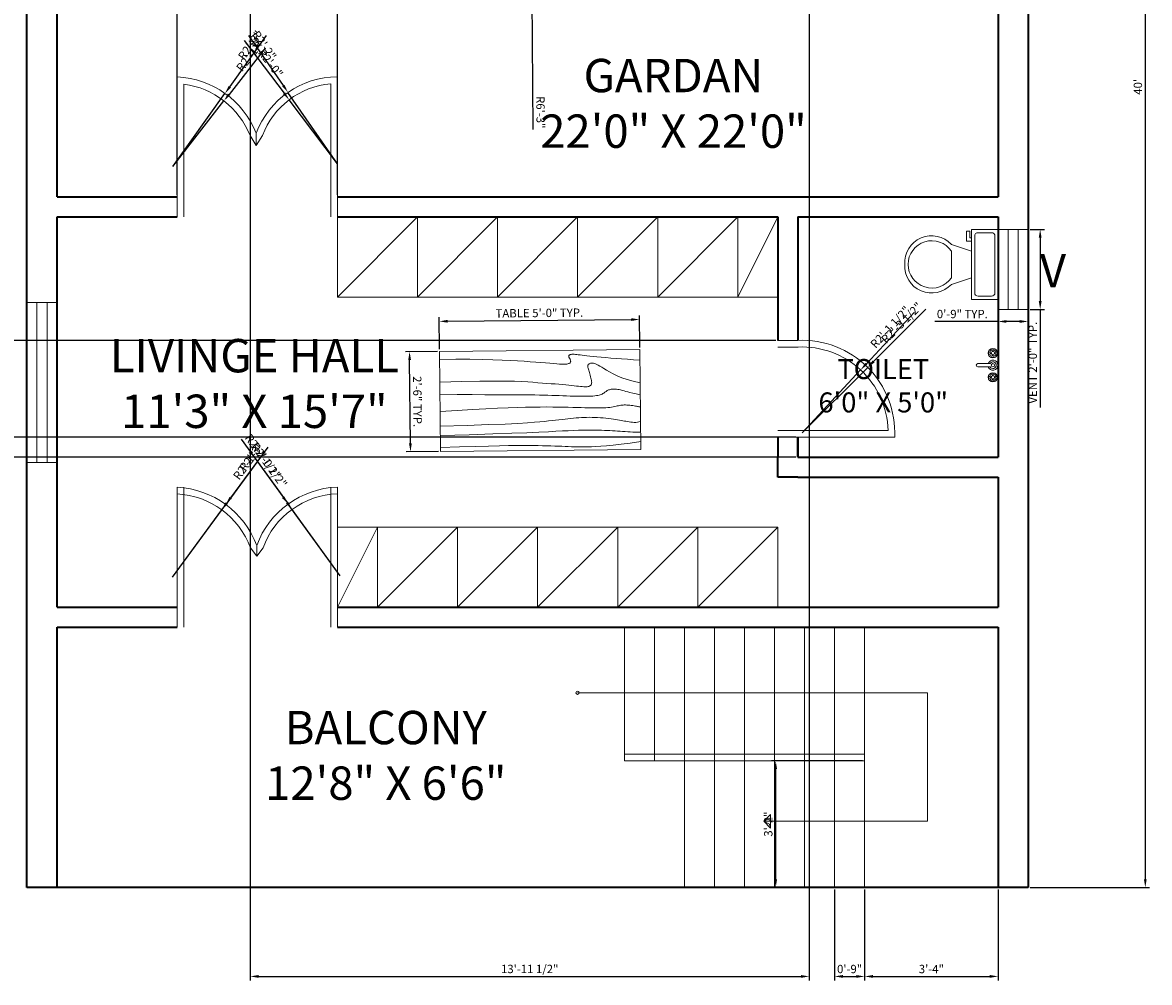
# Model space of a CAD drawing. Units: inches. Extents: x 2318 to 3542, y 1525 to 2117.
# Tile 5 of 6: x 3169 to 3507, y 1529 to 1816. Entities that reach past the tile are written whole.
import ezdxf

# ---------------------------------------------------------------- set-up
doc = ezdxf.new("R2010")
doc.units = ezdxf.units.IN
for name, color, linetype, lineweight in [('A-ANNO-DIMS', 2, 'Continuous', 18), ('A-ANNO-SYMB', 2, 'Continuous', 13), ('A-ANNO-TEXT', 7, 'Continuous', 18), ('A-AREA-IDEN', 7, 'Continuous', 25), ('A-DOOR', 4, 'Continuous', 18), ('A-FLOR-FIXT', 9, 'Continuous', 18), ('A-FLOR-STRS', 3, 'Continuous', 18), ('A-FURN', 8, 'Continuous', 18), ('A-GLAZ', 4, 'Continuous', 18), ('A-WALL', 7, 'Continuous', 35)]:
    doc.layers.add(name, color=color, linetype=linetype, lineweight=lineweight)
doc.styles.add('Annotative', font='arial.ttf')
doc.styles.get("Standard").update_dxf_attribs({"font": 'arial.ttf'})
doc.dimstyles.new('ISO-25', dxfattribs={"dimtxt": 2.5, "dimasz": 2.5, "dimexe": 1.25, "dimexo": 0.625, "dimtad": 1, "dimdec": 0, "dimlunit": 3, "dimtxsty": 'Standard', "dimcen": 2.5, "dimadec": 0, "dimazin": 0, "dimtfac": 1, "dimtdec": 0, "dimtmove": 0, "dimatfit": 3, "dimfxl": 1, "dimarcsym": 0})

# ---------------------------------------------------------------- blocks, each defined once
blk = doc.blocks.new('*D20')
at = {"layer": 'A-ANNO-DIMS', "color": 0, "lineweight": -2, "transparency": 16777216}
for p, q in [((3471.06, 2037.09), (3506.78, 2037.09)), ((3505.53, 2034.59), (3505.53, 1559.59)), ((3471.06, 1557.09), (3506.78, 1557.09))]:
    blk.add_line(p, q, dxfattribs=at)
at = {"layer": 'A-ANNO-DIMS', "color": 0, "transparency": 16777216}
for points in [[(3505.11, 2034.59), (3505.94, 2034.59), (3505.53, 2037.09)], [(3505.11, 1559.59), (3505.94, 1559.59), (3505.53, 1557.09)]]:
    blk.add_solid(points, dxfattribs=at)
at = {"layer": 'Defpoints', "color": 0, "transparency": 16777216}
for p in [(3470.43, 2037.09), (3470.43, 1557.09), (3505.53, 1557.09)]:
    blk.add_point(p, dxfattribs=at)
at = {"layer": 'A-ANNO-DIMS', "color": 0, "transparency": 16777216, "insert": (3503.63, 1797.09), "char_height": 2.5, "attachment_point": 5, "rotation": 90}
blk.add_mtext("40'", dxfattribs=at)
blk = doc.blocks.new('Table - Rectangular Woodgrain 60 x 30 in.')
for p, q in [((0, 0), (0, -30)), ((60, 0), (0, 0)), ((60, -30), (60, 0)), ((0, -30), (60, -30))]:
    blk.add_line(p, q)
for points in [[(0, -2.4), (4.8155, -2.418), (9.0302, -2.4688), (12.709, -2.5477), (15.9167, -2.65), (18.7181, -2.7711), (21.1781, -2.9063), (23.3616, -3.0508), (25.3333, -3.2), (27.1477, -3.3495), (28.8172, -3.4958), (30.3437, -3.636), (31.7291, -3.7667), (32.9756, -3.8849), (34.0849, -3.9875), (35.059, -4.0714), (35.9, -4.1334), (36.6114, -4.1711), (37.2041, -4.1854), (37.6906, -4.1779), (38.0833, -4.15), (38.3948, -4.1034), (38.6375, -4.0396), (38.8239, -3.9602), (38.9666, -3.8667), (39.0764, -3.7608), (39.1573, -3.6448), (39.2116, -3.521), (39.2416, -3.3917), (39.2498, -3.2593), (39.2385, -3.1261), (39.21, -2.9944), (39.1666, -2.8667), (39.111, -2.7447), (39.0468, -2.6281), (38.978, -2.5163), (38.9083, -2.4083), (38.8418, -2.3035), (38.7823, -2.201), (38.7337, -2.1001), (38.7, -2), (38.6844, -1.9003), (38.6875, -1.8021), (38.7094, -1.707), (38.75, -1.6167), (38.8094, -1.5326), (38.8875, -1.4563), (38.9844, -1.3893), (39.1, -1.3333), (39.2351, -1.2896), (39.3937, -1.2583), (39.5804, -1.2396), (39.8, -1.2333), (40.057, -1.2396), (40.3562, -1.2583), (40.7023, -1.2896), (41.1, -1.3333), (41.5547, -1.3895), (42.0755, -1.4573), (42.6721, -1.5361), (43.3542, -1.625), (44.1316, -1.7233), (45.014, -1.8302), (46.0114, -1.9449), (47.1333, -2.0667), (48.3862, -2.1947), (49.7625, -2.3281), (51.2513, -2.4663), (52.8416, -2.6083), (54.5226, -2.7535), (56.2833, -2.9011), (58.1127, -3.0501), (60, -3.2)], [(0, -9.2), (6.5759, -9.0858), (11.9385, -9.0365), (16.2527, -9.0418), (19.6833, -9.0917), (22.3952, -9.1759), (24.5531, -9.2844), (26.322, -9.4069), (27.8666, -9.5333), (29.3241, -9.6553), (30.7203, -9.7719), (32.0532, -9.8837), (33.3208, -9.9917), (34.5213, -10.0965), (35.6526, -10.199), (36.7128, -10.2999), (37.7, -10.4), (38.6129, -10.4996), (39.4531, -10.5969), (40.223, -10.6895), (40.925, -10.775), (41.5613, -10.8512), (42.1344, -10.9156), (42.6465, -10.966), (43.1, -11), (43.4976, -11.0158), (43.8437, -11.0136), (44.143, -10.9942), (44.4, -10.9583), (44.6195, -10.9069), (44.8062, -10.8406), (44.9648, -10.7603), (45.1, -10.6667), (45.2155, -10.5598), (45.3114, -10.4365), (45.3871, -10.2929), (45.4416, -10.125), (45.4743, -9.929), (45.4844, -9.7011), (45.4709, -9.4371), (45.4333, -9.1333), (45.3716, -8.7883), (45.2896, -8.4104), (45.1919, -8.0107), (45.0833, -7.6), (44.9685, -7.1893), (44.8521, -6.7896), (44.7388, -6.4117), (44.6333, -6.0667), (44.54, -5.7628), (44.4614, -5.4979), (44.4001, -5.2675), (44.3583, -5.0667), (44.3384, -4.8909), (44.3427, -4.7354), (44.3736, -4.5956), (44.4333, -4.4667), (44.5236, -4.3453), (44.6427, -4.2333), (44.7884, -4.1339), (44.9583, -4.05), (45.1501, -3.9849), (45.3614, -3.9417), (45.59, -3.9234), (45.8333, -3.9333), (46.0915, -3.9749), (46.3734, -4.0531), (46.6906, -4.1736), (47.0542, -4.3417), (47.4756, -4.5629), (47.9661, -4.8427), (48.5372, -5.1866), (49.2, -5.6), (49.9676, -6.0844), (50.8594, -6.625), (51.8965, -7.2031), (53.1, -7.8), (54.491, -8.3969), (56.0906, -8.975), (57.9199, -9.5156), (60, -10)], [(0, -12.8), (5.1847, -12.9322), (9.6213, -13.0323), (13.3963, -13.1059), (16.5958, -13.1583), (19.3063, -13.1952), (21.614, -13.2219), (23.6054, -13.2439), (25.3666, -13.2667), (26.9728, -13.2947), (28.4531, -13.3281), (29.8256, -13.3663), (31.1083, -13.4083), (32.3191, -13.4535), (33.476, -13.501), (34.597, -13.5501), (35.7, -13.6), (36.7984, -13.6497), (37.8875, -13.6979), (38.9578, -13.743), (40, -13.7833), (41.0047, -13.8174), (41.9625, -13.8438), (42.864, -13.8607), (43.7, -13.8667), (44.4631, -13.8604), (45.1552, -13.8417), (45.7801, -13.8104), (46.3416, -13.7667), (46.8439, -13.7104), (47.2906, -13.6417), (47.6858, -13.5604), (48.0333, -13.4667), (48.3375, -13.3608), (48.6042, -13.2448), (48.8396, -13.121), (49.05, -12.9917), (49.2417, -12.8593), (49.4208, -12.7261), (49.5937, -12.5944), (49.7667, -12.4667), (49.9452, -12.3451), (50.1323, -12.2313), (50.3303, -12.1268), (50.5416, -12.0333), (50.7686, -11.9524), (51.0135, -11.8854), (51.2788, -11.8341), (51.5666, -11.8), (51.8785, -11.7843), (52.2116, -11.7865), (52.562, -11.8059), (52.926, -11.8417), (53.2998, -11.8931), (53.6795, -11.9594), (54.0614, -12.0397), (54.4416, -12.1333), (54.8223, -12.2401), (55.2293, -12.3625), (55.6942, -12.5037), (56.2489, -12.6667), (56.9251, -12.8547), (57.7545, -13.0708), (58.7689, -13.3182), (60, -13.6)], [(0, -18), (5.124, -17.7273), (9.6609, -17.5057), (13.6705, -17.3303), (17.2125, -17.1958), (20.3467, -17.0973), (23.1328, -17.0297), (25.6307, -16.9878), (27.9, -16.9667), (29.9928, -16.9617), (31.9302, -16.9703), (33.7254, -16.9907), (35.3917, -17.0208), (36.9423, -17.0588), (38.3906, -17.1026), (39.7499, -17.1503), (41.0333, -17.2), (42.2519, -17.2496), (43.4073, -17.2969), (44.4986, -17.3395), (45.525, -17.375), (46.4858, -17.4012), (47.3802, -17.4156), (48.2074, -17.416), (48.9667, -17.4), (49.6583, -17.3662), (50.2872, -17.3167), (50.8595, -17.2547), (51.3812, -17.1833), (51.8584, -17.1057), (52.2971, -17.025), (52.7034, -16.9443), (53.0833, -16.8667), (53.443, -16.7951), (53.789, -16.7313), (54.128, -16.6768), (54.4666, -16.6334), (54.8115, -16.6024), (55.1693, -16.5854), (55.5465, -16.5841), (55.95, -16.6), (56.3828, -16.6337), (56.8346, -16.6823), (57.2915, -16.7418), (57.7396, -16.8084), (58.165, -16.878), (58.5539, -16.9469), (58.8924, -17.0111), (59.1666, -17.0667), (59.3679, -17.1107), (59.5078, -17.1438), (59.6032, -17.1675), (59.6708, -17.1833), (59.7275, -17.193), (59.7901, -17.1979), (59.8753, -17.1998), (60, -17.2)], [(0, -22.4), (8.0098, -22.2501), (14.4094, -22.1011), (19.4168, -21.9535), (23.25, -21.8083), (26.1269, -21.6663), (28.2656, -21.5281), (29.884, -21.3947), (31.2, -21.2667), (32.3967, -21.1448), (33.5172, -21.0292), (34.5697, -20.9198), (35.5625, -20.8167), (36.5037, -20.7198), (37.4015, -20.6292), (38.2642, -20.5448), (39.1, -20.4667), (39.9164, -20.3951), (40.7187, -20.3313), (41.5117, -20.2768), (42.3, -20.2333), (43.0883, -20.2024), (43.8812, -20.1854), (44.6836, -20.1841), (45.5, -20.2), (46.3328, -20.234), (47.1747, -20.2844), (48.0163, -20.3488), (48.8479, -20.425), (49.66, -20.5106), (50.4429, -20.6031), (51.1872, -20.7004), (51.8833, -20.8), (52.5246, -20.8999), (53.1166, -20.9995), (53.6681, -21.0983), (54.1875, -21.1958), (54.6834, -21.2919), (55.1646, -21.3859), (55.6394, -21.4777), (56.1167, -21.5667), (56.6028, -21.6515), (57.0961, -21.7266), (57.5929, -21.7852), (58.0896, -21.8208), (58.5823, -21.8268), (59.0674, -21.7964), (59.5412, -21.723), (60, -21.6)], [(0, -25.2), (8.6355, -25.0504), (15.7026, -24.9031), (21.4049, -24.7606), (25.9458, -24.625), (29.529, -24.4988), (32.3578, -24.3844), (34.6359, -24.284), (36.5667, -24.2), (38.3213, -24.1341), (39.9417, -24.0854), (41.437, -24.0523), (42.8167, -24.0333), (44.0901, -24.0268), (45.2667, -24.0313), (46.3557, -24.0451), (47.3667, -24.0667), (48.309, -24.0947), (49.1928, -24.1287), (50.0284, -24.168), (50.826, -24.2125), (51.5959, -24.2617), (52.3483, -24.3151), (53.0935, -24.3725), (53.8417, -24.4334), (54.6009, -24.497), (55.3699, -24.561), (56.1454, -24.6226), (56.9239, -24.6792), (57.7021, -24.7279), (58.4764, -24.7662), (59.2435, -24.7911), (60, -24.8)], [(0, -28.8), (5.6867, -28.6681), (10.45, -28.5698), (14.407, -28.5012), (17.675, -28.4584), (20.3711, -28.4374), (22.6125, -28.4344), (24.5164, -28.4455), (26.2, -28.4667), (27.762, -28.4947), (29.2276, -28.5281), (30.6033, -28.5663), (31.8958, -28.6084), (33.1118, -28.6535), (34.2578, -28.7011), (35.3405, -28.7501), (36.3666, -28.8), (37.3443, -28.8497), (38.288, -28.8974), (39.2137, -28.9412), (40.1375, -28.9792), (41.0753, -29.0093), (42.0432, -29.0297), (43.0572, -29.0384), (44.1333, -29.0333), (45.2936, -29.0114), (46.5843, -28.9641), (48.0579, -28.8816), (49.7666, -28.7542), (51.7629, -28.5721), (54.0989, -28.3255), (56.8272, -28.0048), (60, -27.6)]]:
    blk.add_lwpolyline(points)
blk = doc.blocks.new('*U14')
for p, q in [((241.3, -152.4), (241.3, -50.8)), ((-254, -215.9), (-203.2, -215.9)), ((-254, -241.3), (-254, -215.9)), ((-177.8, -241.3), (-254, -241.3)), ((-203.2, -215.9), (-203.2, -203.2)), ((-177.8, -203.2), (-177.8, -241.3)), ((-101.6, -203.2), (-152.4, -355.6)), ((101.6, -203.2), (152.4, -355.6)), ((101.6, -355.6), (-101.6, -355.6))]:
    blk.add_line(p, q)
blk.add_lwpolyline([(266.7, -203.2), (266.7, 0), (-266.7, 0), (-266.7, -203.2)], close=True)
for points in [[(-241.3, -50.8), (-241.3, -152.4)], [(215.9, -25.4), (-215.9, -25.4)], [(-215.9, -177.8), (215.9, -177.8)]]:
    blk.add_lwpolyline(points)
for centre, radius, start, end in [((-219.075, -47.625), 22.45064, 81.8699, 188.1301), ((219.075, -47.625), 22.45064, 351.8699, 98.1301), ((-219.075, -155.575), 22.45064, 171.869898, 278.1301), ((219.075, -155.575), 22.45064, 261.8699, 8.1301), ((-12.12088, -505.93752), 205.61935, 133.01722, 273.38), ((0.94996, -504.77674), 181.02486, 124.50543, 269.7), ((-0.94742, -504.77674), 181.02486, 270.3, 55.4946), ((12.12342, -505.93752), 205.61935, 266.62, 46.9828)]:
    blk.add_arc(centre, radius, start, end)
blk = doc.blocks.new('Faucet - Bathroom top')
for p, q in [((-4.107, 0.125), (-4.375, 0.125)), ((-3.75, 0.4788), (-3.75, 0.75)), ((-3.5, 0.482), (-3.5, 0.75)), ((-3.1461, 0.125), (-2.875, 0.125)), ((3.143, 0.125), (2.875, 0.125)), ((3.5, 0.4788), (3.5, 0.75)), ((3.75, 0.482), (3.75, 0.75)), ((4.1039, 0.125), (4.375, 0.125)), ((-4.1039, -0.125), (-4.375, -0.125)), ((-3.75, -0.4821), (-3.75, -0.75)), ((-3.5, -0.4789), (-3.5, -0.75)), ((-3.143, -0.125), (-2.875, -0.125)), ((-0.5, -0.8639), (-0.5, -4.5)), ((0.5, -4.5), (0.5, -0.8631)), ((3.1461, -0.125), (2.875, -0.125)), ((3.5, -0.4821), (3.5, -0.75)), ((3.75, -0.4789), (3.75, -0.75)), ((4.107, -0.125), (4.375, -0.125))]:
    blk.add_line(p, q)
for centre, radius in [((-3.625, 0), 1.375), ((-4.625, 0), 0.2795), ((-3.625, 0), 0.5), ((-3.625, 1), 0.2795), ((-2.625, 0), 0.2795), ((0, 0), 0.5), ((3.625, 0), 1.375), ((2.625, 0), 0.2795), ((3.625, 0), 0.5), ((3.625, 1), 0.2795), ((4.625, 0), 0.2795), ((-3.625, -1), 0.2795), ((3.625, -1), 0.2795)]:
    blk.add_circle(centre, radius)
for centre, radius, start, end in [((-3.625, 0), 1, 105.2407, 164.2093), ((-3.625, 0), 1, 16.44125, 74.07887), ((0, 0), 1.5, 289.6514, 250.3603), ((0, 0), 1, 300.3431, 239.7554), ((3.625, 0), 1, 106.12, 164.0884), ((3.625, 0), 1, 16.23422, 73.90469), ((-3.625, 0), 1, 196.2342, 253.9047), ((-3.625, 0), 1, 286.12, 344.0884), ((3.625, 0), 1, 196.4413, 254.0789), ((3.625, 0), 1, 285.2407, 344.2093), ((0, -4.5), 0.5, 180, 0)]:
    blk.add_arc(centre, radius, start, end)
blk = doc.blocks.new('WIN-48x9')
for p, q in [((48, 9), (0, 9)), ((0, 9), (0, 0)), ((48, 0), (48, 9)), ((48, 6), (0, 6)), ((0, 3), (48, 3)), ((0, 0), (48, 0))]:
    blk.add_line(p, q)
blk = doc.blocks.new('VENT-24x9')
for p, q in [((0, 24), (0, 0)), ((9, 24), (0, 24)), ((3, 24), (3, 0)), ((6, 0), (6, 24)), ((9, 0), (9, 24)), ((0, 0), (9, 0))]:
    blk.add_line(p, q)
blk = doc.blocks.new('STAIR-ARROWHEAD')
for p, q in [((0, 2), (2, 4)), ((2, 2), (2, 4)), ((2, 4), (2, 2)), ((2, 4), (2, 0)), ((0, 2), (2, 3)), ((2, 2), (0, 2)), ((2, 0), (0, 2)), ((2, 1), (0, 2)), ((2, 3), (2, 1)), ((2, 2), (2, 0)), ((2, 0), (2, 2))]:
    blk.add_line(p, q)
blk = doc.blocks.new('*D34')
at = {"layer": 'A-ANNO-DIMS', "color": 0, "lineweight": -2, "transparency": 16777216}
for p, q in [((3471.06, 1754.36), (3475.28, 1754.36)), ((3474.03, 1751.86), (3474.03, 1732.86)), ((3471.06, 1730.36), (3475.28, 1730.36)), ((3474.03, 1730.36), (3474.03, 1700.96))]:
    blk.add_line(p, q, dxfattribs=at)
at = {"layer": 'A-ANNO-DIMS', "color": 0, "transparency": 16777216}
for points in [[(3473.61, 1751.86), (3474.45, 1751.86), (3474.03, 1754.36)], [(3473.61, 1732.86), (3474.45, 1732.86), (3474.03, 1730.36)]]:
    blk.add_solid(points, dxfattribs=at)
at = {"layer": 'Defpoints', "color": 0, "transparency": 16777216}
for p in [(3470.43, 1754.36), (3470.43, 1730.36), (3474.03, 1730.36)]:
    blk.add_point(p, dxfattribs=at)
at = {"layer": 'A-ANNO-DIMS', "color": 0, "transparency": 16777216, "insert": (3472.13, 1714.41), "char_height": 2.5, "attachment_point": 5, "rotation": 90}
blk.add_mtext('VENT 2\'-0" TYP.', dxfattribs=at)
blk = doc.blocks.new('*D35')
at = {"layer": 'A-ANNO-DIMS', "color": 0, "lineweight": -2, "transparency": 16777216}
for p, q in [((3461.43, 1729.74), (3461.43, 1725.51)), ((3470.43, 1729.74), (3470.43, 1725.51)), ((3461.43, 1726.76), (3442.44, 1726.76)), ((3467.93, 1726.76), (3463.93, 1726.76))]:
    blk.add_line(p, q, dxfattribs=at)
at = {"layer": 'A-ANNO-DIMS', "color": 0, "transparency": 16777216}
for points in [[(3463.93, 1727.18), (3463.93, 1726.35), (3461.43, 1726.76)], [(3467.93, 1727.18), (3467.93, 1726.35), (3470.43, 1726.76)]]:
    blk.add_solid(points, dxfattribs=at)
at = {"layer": 'Defpoints', "color": 0, "transparency": 16777216}
for p in [(3461.43, 1730.36), (3470.43, 1730.36), (3461.43, 1726.76)]:
    blk.add_point(p, dxfattribs=at)
at = {"layer": 'A-ANNO-DIMS', "color": 0, "transparency": 16777216, "insert": (3450.69, 1728.67), "char_height": 2.5, "attachment_point": 5}
blk.add_mtext('0\'-9" TYP.', dxfattribs=at)
blk = doc.blocks.new('*D44')
at = {"layer": 'A-ANNO-DIMS', "color": 0, "lineweight": -2, "transparency": 16777216}
for p, q in [((3294.06, 1718.42), (3293.97, 1728.05)), ((3296.48, 1726.82), (3351.48, 1727.33)), ((3354.06, 1718.98), (3353.97, 1728.6))]:
    blk.add_line(p, q, dxfattribs=at)
at = {"layer": 'A-ANNO-DIMS', "color": 0, "transparency": 16777216}
for points in [[(3296.48, 1727.24), (3296.49, 1726.4), (3293.98, 1726.8)], [(3351.48, 1727.75), (3351.48, 1726.91), (3353.98, 1727.35)]]:
    blk.add_solid(points, dxfattribs=at)
at = {"layer": 'Defpoints', "color": 0, "transparency": 16777216}
for p in [(3353.98, 1727.35), (3294.07, 1717.8), (3354.06, 1718.35)]:
    blk.add_point(p, dxfattribs=at)
at = {"layer": 'A-ANNO-DIMS', "color": 0, "transparency": 16777216, "insert": (3323.96, 1728.98), "char_height": 2.5, "attachment_point": 5, "rotation": 0.5327}
blk.add_mtext('TABLE 5\'-0" TYP.', dxfattribs=at)
blk = doc.blocks.new('*D45')
at = {"layer": 'A-ANNO-DIMS', "color": 0, "lineweight": -2, "transparency": 16777216}
for p, q in [((3293.44, 1717.79), (3283.82, 1717.7)), ((3285.32, 1690.21), (3285.09, 1715.21)), ((3293.72, 1687.79), (3284.1, 1687.7))]:
    blk.add_line(p, q, dxfattribs=at)
at = {"layer": 'A-ANNO-DIMS', "color": 0, "transparency": 16777216}
for points in [[(3285.51, 1715.22), (3284.67, 1715.21), (3285.07, 1717.71)], [(3285.74, 1690.22), (3284.91, 1690.21), (3285.35, 1687.71)]]:
    blk.add_solid(points, dxfattribs=at)
at = {"layer": 'Defpoints', "color": 0, "transparency": 16777216}
for p in [(3285.07, 1717.71), (3294.07, 1717.8), (3294.35, 1687.8)]:
    blk.add_point(p, dxfattribs=at)
at = {"layer": 'A-ANNO-DIMS', "color": 0, "transparency": 16777216, "insert": (3287.11, 1702.73), "char_height": 2.5, "attachment_point": 5, "rotation": 270.5327}
blk.add_mtext('2\'-6" TYP.', dxfattribs=at)
blk = doc.blocks.new('*D53')
at = {"layer": 'A-ANNO-DIMS', "color": 0, "lineweight": -2, "transparency": 16777216}
for p, q in [((3237.33, 1838.64), (3237.33, 1529.19)), ((3404.83, 1824.73), (3404.83, 1529.19)), ((3239.83, 1530.44), (3402.33, 1530.44))]:
    blk.add_line(p, q, dxfattribs=at)
at = {"layer": 'A-ANNO-DIMS', "color": 0, "transparency": 16777216}
for points in [[(3239.83, 1530.86), (3239.83, 1530.02), (3237.33, 1530.44)], [(3402.33, 1530.86), (3402.33, 1530.02), (3404.83, 1530.44)]]:
    blk.add_solid(points, dxfattribs=at)
at = {"layer": 'Defpoints', "color": 0, "transparency": 16777216}
for p in [(3237.33, 1839.27), (3404.83, 1825.36), (3404.83, 1530.44)]:
    blk.add_point(p, dxfattribs=at)
at = {"layer": 'A-ANNO-DIMS', "color": 0, "transparency": 16777216, "insert": (3321.08, 1532.36), "char_height": 2.5, "attachment_point": 5}
blk.add_mtext('13\'-11 1/2"', dxfattribs=at)
blk = doc.blocks.new('*D61')
at = {"layer": 'A-ANNO-DIMS', "color": 0, "lineweight": -2, "transparency": 16777216}
for p, q in [((3215.43, 1764.71), (3215.43, 2114.76)), ((3263.43, 1764.71), (3263.43, 2114.76)), ((3217.93, 2113.51), (3260.93, 2113.51))]:
    blk.add_line(p, q, dxfattribs=at)
at = {"layer": 'A-ANNO-DIMS', "color": 0, "transparency": 16777216}
for points in [[(3217.93, 2113.93), (3217.93, 2113.1), (3215.43, 2113.51)], [(3260.93, 2113.93), (3260.93, 2113.1), (3263.43, 2113.51)]]:
    blk.add_solid(points, dxfattribs=at)
at = {"layer": 'Defpoints', "color": 0, "transparency": 16777216}
for p in [(3263.43, 2113.51), (3215.43, 1764.09), (3263.43, 1764.09)]:
    blk.add_point(p, dxfattribs=at)
at = {"layer": 'A-ANNO-DIMS', "color": 0, "transparency": 16777216, "insert": (3239.43, 2115.41), "char_height": 2.5, "attachment_point": 5}
blk.add_mtext('4\'-0"', dxfattribs=at)
blk = doc.blocks.new('*D64')
at = {"layer": 'A-ANNO-DIMS', "color": 0, "lineweight": -2, "transparency": 16777216}
for p, q in [((3394.81, 1721.09), (3104.01, 1721.09)), ((3105.26, 1694.59), (3105.26, 1718.59)), ((3394.81, 1692.09), (3104.01, 1692.09))]:
    blk.add_line(p, q, dxfattribs=at)
at = {"layer": 'A-ANNO-DIMS', "color": 0, "transparency": 16777216}
for points in [[(3104.85, 1718.59), (3105.68, 1718.59), (3105.26, 1721.09)], [(3104.85, 1694.59), (3105.68, 1694.59), (3105.26, 1692.09)]]:
    blk.add_solid(points, dxfattribs=at)
at = {"layer": 'Defpoints', "color": 0, "transparency": 16777216}
for p in [(3105.26, 1721.09), (3395.43, 1721.09), (3395.43, 1692.09)]:
    blk.add_point(p, dxfattribs=at)
at = {"layer": 'A-ANNO-DIMS', "color": 0, "transparency": 16777216, "insert": (3103.36, 1706.59), "char_height": 2.5, "attachment_point": 5, "rotation": 90}
blk.add_mtext('2\'-5"', dxfattribs=at)
blk = doc.blocks.new('*D65')
at = {"layer": 'A-ANNO-DIMS', "color": 0, "lineweight": -2, "transparency": 16777216}
for p, q in [((3105.26, 1694.59), (3105.26, 1704.98)), ((3400.81, 1692.09), (3104.01, 1692.09)), ((3105.26, 1686.09), (3105.26, 1692.09)), ((3400.81, 1686.09), (3104.01, 1686.09)), ((3105.26, 1683.59), (3105.26, 1681.09))]:
    blk.add_line(p, q, dxfattribs=at)
at = {"layer": 'A-ANNO-DIMS', "color": 0, "transparency": 16777216}
for points in [[(3104.85, 1694.59), (3105.68, 1694.59), (3105.26, 1692.09)], [(3104.85, 1683.59), (3105.68, 1683.59), (3105.26, 1686.09)]]:
    blk.add_solid(points, dxfattribs=at)
at = {"layer": 'Defpoints', "color": 0, "transparency": 16777216}
for p in [(3105.26, 1692.09), (3401.43, 1692.09), (3401.43, 1686.09)]:
    blk.add_point(p, dxfattribs=at)
at = {"layer": 'A-ANNO-DIMS', "color": 0, "transparency": 16777216, "insert": (3103.36, 1701.04), "char_height": 2.5, "attachment_point": 5, "rotation": 90}
blk.add_mtext('0\'-6"', dxfattribs=at)
blk = doc.blocks.new('*D68')
at = {"layer": 'A-ANNO-DIMS', "color": 0, "lineweight": -2, "transparency": 16777216}
for p, q in [((3420.81, 1595.09), (3393.53, 1595.09)), ((3394.78, 1559.59), (3394.78, 1592.59)), ((3420.81, 1557.09), (3393.53, 1557.09))]:
    blk.add_line(p, q, dxfattribs=at)
at = {"layer": 'A-ANNO-DIMS', "color": 0, "transparency": 16777216}
for points in [[(3394.36, 1592.59), (3395.2, 1592.59), (3394.78, 1595.09)], [(3394.36, 1559.59), (3395.2, 1559.59), (3394.78, 1557.09)]]:
    blk.add_solid(points, dxfattribs=at)
at = {"layer": 'Defpoints', "color": 0, "transparency": 16777216}
for p in [(3394.78, 1595.09), (3421.43, 1595.09), (3421.43, 1557.09)]:
    blk.add_point(p, dxfattribs=at)
at = {"layer": 'A-ANNO-DIMS', "color": 0, "transparency": 16777216, "insert": (3392.88, 1576.09), "char_height": 2.5, "attachment_point": 5, "rotation": 90}
blk.add_mtext('3\'-2"', dxfattribs=at)
blk = doc.blocks.new('*D69')
at = {"layer": 'A-ANNO-DIMS', "color": 0, "lineweight": -2, "transparency": 16777216}
for p, q in [((3412.43, 1556.46), (3412.43, 1529.19)), ((3421.43, 1556.46), (3421.43, 1529.19)), ((3414.93, 1530.44), (3418.93, 1530.44))]:
    blk.add_line(p, q, dxfattribs=at)
at = {"layer": 'A-ANNO-DIMS', "color": 0, "transparency": 16777216}
for points in [[(3414.93, 1530.86), (3414.93, 1530.02), (3412.43, 1530.44)], [(3418.93, 1530.86), (3418.93, 1530.02), (3421.43, 1530.44)]]:
    blk.add_solid(points, dxfattribs=at)
at = {"layer": 'Defpoints', "color": 0, "transparency": 16777216}
for p in [(3412.43, 1557.09), (3421.43, 1557.09), (3421.43, 1530.44)]:
    blk.add_point(p, dxfattribs=at)
at = {"layer": 'A-ANNO-DIMS', "color": 0, "transparency": 16777216, "insert": (3416.93, 1532.34), "char_height": 2.5, "attachment_point": 5}
blk.add_mtext('0\'-9"', dxfattribs=at)
blk = doc.blocks.new('*D70')
at = {"layer": 'A-ANNO-DIMS', "color": 0, "lineweight": -2, "transparency": 16777216}
for p, q in [((3421.43, 1556.46), (3421.43, 1529.19)), ((3461.43, 1556.46), (3461.43, 1529.19)), ((3423.93, 1530.44), (3458.93, 1530.44))]:
    blk.add_line(p, q, dxfattribs=at)
at = {"layer": 'A-ANNO-DIMS', "color": 0, "transparency": 16777216}
for points in [[(3423.93, 1530.86), (3423.93, 1530.02), (3421.43, 1530.44)], [(3458.93, 1530.86), (3458.93, 1530.02), (3461.43, 1530.44)]]:
    blk.add_solid(points, dxfattribs=at)
at = {"layer": 'Defpoints', "color": 0, "transparency": 16777216}
for p in [(3421.43, 1557.09), (3461.43, 1557.09), (3461.43, 1530.44)]:
    blk.add_point(p, dxfattribs=at)
at = {"layer": 'A-ANNO-DIMS', "color": 0, "transparency": 16777216, "insert": (3441.43, 1532.34), "char_height": 2.5, "attachment_point": 5}
blk.add_mtext('3\'-4"', dxfattribs=at)
blk = doc.blocks.new('*D86')
at = {"layer": 'A-ANNO-DIMS', "color": 0, "lineweight": -2, "transparency": 16777216}
for p, q in [((3439.8, 1730.46), (3424.11, 1714.77)), ((3402.73, 1693.39), (3422.34, 1713))]:
    blk.add_line(p, q, dxfattribs=at)
at = {"layer": 'A-ANNO-DIMS', "color": 0, "transparency": 16777216}
blk.add_solid([(3423.81, 1715.06), (3424.4, 1714.47), (3422.34, 1713)], dxfattribs=at)
at = {"layer": 'Defpoints', "color": 0, "transparency": 16777216}
for p in [(3422.34, 1713), (3402.73, 1693.39)]:
    blk.add_point(p, dxfattribs=at)
at = {"layer": 'A-ANNO-DIMS', "color": 0, "transparency": 16777216, "insert": (3432.75, 1726.12), "char_height": 2.5, "attachment_point": 5, "rotation": 45.0003}
blk.add_mtext('R2\'-3 1/2"', dxfattribs=at)
blk = doc.blocks.new('*D92')
at = {"layer": 'A-ANNO-DIMS', "color": 0, "lineweight": -2, "transparency": 16777216}
for p, q in [((3242.11, 1812.45), (3231.21, 1797.16)), ((3214.15, 1773.23), (3229.75, 1795.13))]:
    blk.add_line(p, q, dxfattribs=at)
at = {"layer": 'A-ANNO-DIMS', "color": 0, "transparency": 16777216}
blk.add_solid([(3230.87, 1797.4), (3231.55, 1796.92), (3229.75, 1795.13)], dxfattribs=at)
at = {"layer": 'Defpoints', "color": 0, "transparency": 16777216}
for p in [(3229.75, 1795.13), (3214.15, 1773.23)]:
    blk.add_point(p, dxfattribs=at)
at = {"layer": 'A-ANNO-DIMS', "color": 0, "transparency": 16777216, "insert": (3237.57, 1809.37), "char_height": 2.5, "attachment_point": 5, "rotation": 54.5145}
blk.add_mtext('R2\'-3"', dxfattribs=at)
blk = doc.blocks.new('*D93')
at = {"layer": 'A-ANNO-DIMS', "color": 0, "lineweight": -2, "transparency": 16777216}
for p, q in [((3236.79, 1812.5), (3247.22, 1797.49)), ((3263.5, 1774.04), (3248.64, 1795.44))]:
    blk.add_line(p, q, dxfattribs=at)
at = {"layer": 'A-ANNO-DIMS', "color": 0, "transparency": 16777216}
blk.add_solid([(3247.56, 1797.73), (3246.87, 1797.25), (3248.64, 1795.44)], dxfattribs=at)
at = {"layer": 'Defpoints', "color": 0, "transparency": 16777216}
for p in [(3248.64, 1795.44), (3263.5, 1774.04)]:
    blk.add_point(p, dxfattribs=at)
at = {"layer": 'A-ANNO-DIMS', "color": 0, "transparency": 16777216, "insert": (3241.27, 1809.34), "char_height": 2.5, "attachment_point": 5, "rotation": 304.7777}
blk.add_mtext('R2\'-2"', dxfattribs=at)
blk = doc.blocks.new('*D94')
at = {"layer": 'A-ANNO-DIMS', "color": 0, "lineweight": -2, "transparency": 16777216}
for p, q in [((3242.59, 1689.1), (3231.45, 1673.92)), ((3214.02, 1650.15), (3229.97, 1671.9))]:
    blk.add_line(p, q, dxfattribs=at)
at = {"layer": 'A-ANNO-DIMS', "color": 0, "transparency": 16777216}
blk.add_solid([(3231.12, 1674.17), (3231.79, 1673.67), (3229.97, 1671.9)], dxfattribs=at)
at = {"layer": 'Defpoints', "color": 0, "transparency": 16777216}
for p in [(3229.97, 1671.9), (3214.02, 1650.15)]:
    blk.add_point(p, dxfattribs=at)
at = {"layer": 'A-ANNO-DIMS', "color": 0, "transparency": 16777216, "insert": (3238.01, 1686.08), "char_height": 2.5, "attachment_point": 5, "rotation": 53.7455}
blk.add_mtext('R2\'-3"', dxfattribs=at)
blk = doc.blocks.new('*D95')
at = {"layer": 'A-ANNO-DIMS', "color": 0, "lineweight": -2, "transparency": 16777216}
for p, q in [((3234.59, 1691.48), (3247.21, 1674.07)), ((3264.27, 1650.53), (3248.68, 1672.04))]:
    blk.add_line(p, q, dxfattribs=at)
at = {"layer": 'A-ANNO-DIMS', "color": 0, "transparency": 16777216}
blk.add_solid([(3247.55, 1674.31), (3246.87, 1673.82), (3248.68, 1672.04)], dxfattribs=at)
at = {"layer": 'Defpoints', "color": 0, "transparency": 16777216}
for p in [(3248.68, 1672.04), (3264.27, 1650.53)]:
    blk.add_point(p, dxfattribs=at)
at = {"layer": 'A-ANNO-DIMS', "color": 0, "transparency": 16777216, "insert": (3240.87, 1686.08), "char_height": 2.5, "attachment_point": 5, "rotation": 305.9363}
blk.add_mtext('R2\'-2 1/2"', dxfattribs=at)
blk = doc.blocks.new('*D102')
at = {"layer": 'A-ANNO-DIMS', "color": 0, "lineweight": -2, "transparency": 16777216}
for p, q in [((3436.23, 1729.46), (3421.94, 1714.08)), ((3402.73, 1693.39), (3420.24, 1712.24))]:
    blk.add_line(p, q, dxfattribs=at)
at = {"layer": 'A-ANNO-DIMS', "color": 0, "transparency": 16777216}
blk.add_solid([(3421.63, 1714.36), (3422.25, 1713.79), (3420.24, 1712.24)], dxfattribs=at)
at = {"layer": 'Defpoints', "color": 0, "transparency": 16777216}
for p in [(3420.24, 1712.24), (3402.73, 1693.39)]:
    blk.add_point(p, dxfattribs=at)
at = {"layer": 'A-ANNO-DIMS', "color": 0, "transparency": 16777216, "insert": (3429.34, 1724.86), "char_height": 2.5, "attachment_point": 5, "rotation": 47.1232}
blk.add_mtext('R2\'-1 1/2"', dxfattribs=at)
blk = doc.blocks.new('*D103')
at = {"layer": 'A-ANNO-DIMS', "color": 0, "lineweight": -2, "transparency": 16777216}
for p, q in [((3240.7, 1686.52), (3230.27, 1672.31)), ((3214.02, 1650.15), (3228.79, 1670.29))]:
    blk.add_line(p, q, dxfattribs=at)
at = {"layer": 'A-ANNO-DIMS', "color": 0, "transparency": 16777216}
blk.add_solid([(3229.93, 1672.55), (3230.61, 1672.06), (3228.79, 1670.29)], dxfattribs=at)
at = {"layer": 'Defpoints', "color": 0, "transparency": 16777216}
for p in [(3228.79, 1670.29), (3214.02, 1650.15)]:
    blk.add_point(p, dxfattribs=at)
at = {"layer": 'A-ANNO-DIMS', "color": 0, "transparency": 16777216, "insert": (3236.14, 1683.49), "char_height": 2.5, "attachment_point": 5, "rotation": 53.7439}
blk.add_mtext('R2\'-1"', dxfattribs=at)
blk = doc.blocks.new('*D105')
at = {"layer": 'A-ANNO-DIMS', "color": 0, "lineweight": -2, "transparency": 16777216}
for p, q in [((3235.51, 1810.96), (3247.46, 1795.2)), ((3263.5, 1774.04), (3248.97, 1793.2))]:
    blk.add_line(p, q, dxfattribs=at)
at = {"layer": 'A-ANNO-DIMS', "color": 0, "transparency": 16777216}
blk.add_solid([(3247.79, 1795.45), (3247.13, 1794.94), (3248.97, 1793.2)], dxfattribs=at)
at = {"layer": 'Defpoints', "color": 0, "transparency": 16777216}
for p in [(3248.97, 1793.2), (3263.5, 1774.04)]:
    blk.add_point(p, dxfattribs=at)
at = {"layer": 'A-ANNO-DIMS', "color": 0, "transparency": 16777216, "insert": (3241.77, 1805.85), "char_height": 2.5, "attachment_point": 5, "rotation": 307.1715}
blk.add_mtext('2X R2\'-0"', dxfattribs=at)
blk = doc.blocks.new('*D112')
at = {"layer": 'A-ANNO-DIMS', "color": 0, "lineweight": -2, "transparency": 16777216}
for p, q in [((3241.77, 1808.71), (3230.97, 1794.84)), ((3214.15, 1773.23), (3229.44, 1792.87))]:
    blk.add_line(p, q, dxfattribs=at)
at = {"layer": 'A-ANNO-DIMS', "color": 0, "transparency": 16777216}
blk.add_solid([(3230.64, 1795.1), (3231.3, 1794.59), (3229.44, 1792.87)], dxfattribs=at)
at = {"layer": 'Defpoints', "color": 0, "transparency": 16777216}
for p in [(3229.44, 1792.87), (3214.15, 1773.23)]:
    blk.add_point(p, dxfattribs=at)
at = {"layer": 'A-ANNO-DIMS', "color": 0, "transparency": 16777216, "insert": (3237.13, 1805.81), "char_height": 2.5, "attachment_point": 5, "rotation": 52.0935}
blk.add_mtext('R2\'-1"', dxfattribs=at)
blk = doc.blocks.new('*D113')
at = {"layer": 'A-ANNO-DIMS', "color": 0, "lineweight": -2, "transparency": 16777216}
for p, q in [((3236.47, 1688.89), (3248.38, 1672.45)), ((3264.27, 1650.53), (3249.85, 1670.43))]:
    blk.add_line(p, q, dxfattribs=at)
at = {"layer": 'A-ANNO-DIMS', "color": 0, "transparency": 16777216}
blk.add_solid([(3248.72, 1672.69), (3248.04, 1672.21), (3249.85, 1670.43)], dxfattribs=at)
at = {"layer": 'Defpoints', "color": 0, "transparency": 16777216}
for p in [(3249.85, 1670.43), (3264.27, 1650.53)]:
    blk.add_point(p, dxfattribs=at)
at = {"layer": 'A-ANNO-DIMS', "color": 0, "transparency": 16777216, "insert": (3242.75, 1683.49), "char_height": 2.5, "attachment_point": 5, "rotation": 305.9355}
blk.add_mtext('R2\'-0 1/2"', dxfattribs=at)
blk = doc.blocks.new('*D114')
at = {"layer": 'A-ANNO-DIMS', "color": 0, "lineweight": -2, "transparency": 16777216}
for p, q in [((3321.1, 1909.07), (3321.72, 1834.3)), ((3322.14, 1784.3), (3321.74, 1831.8))]:
    blk.add_line(p, q, dxfattribs=at)
at = {"layer": 'A-ANNO-DIMS', "color": 0, "transparency": 16777216}
blk.add_solid([(3322.16, 1831.81), (3321.33, 1831.8), (3321.72, 1834.3)], dxfattribs=at)
at = {"layer": 'Defpoints', "color": 0, "transparency": 16777216}
for p in [(3321.1, 1909.07), (3321.72, 1834.3)]:
    blk.add_point(p, dxfattribs=at)
at = {"layer": 'A-ANNO-DIMS', "color": 0, "transparency": 16777216, "insert": (3324, 1789.46), "char_height": 2.5, "attachment_point": 5, "rotation": 270.4791}
blk.add_mtext('R6\'-3"', dxfattribs=at)

msp = doc.modelspace()

# ---------------------------------------------------------------- linework, layer by layer
at = {"layer": 'A-ANNO-SYMB'}
for p, q in [((3239.12, 1783.2), (3239.12, 1779.55)), ((3239.12, 1779.55), (3237.26, 1782.46)), ((3239.12, 1779.55), (3240.99, 1782.5)), ((3240.99, 1782.5), (3239.12, 1779.55)), ((3239.29, 1656.38), (3237.42, 1658.89)), ((3239.29, 1659.59), (3239.29, 1656.38)), ((3239.29, 1656.38), (3241.17, 1658.91)), ((3241.17, 1658.91), (3239.29, 1656.38)), ((3335.41, 1615.48), (3440.23, 1615.48)), ((3440.23, 1615.48), (3440.23, 1576.93)), ((3440.23, 1576.93), (3393.21, 1576.93)), ((3393.21, 1576.93), (3393.21, 1576.93))]:
    msp.add_line(p, q, dxfattribs=at)
msp.add_circle((3335.41, 1615.48), 0.505, dxfattribs=at)
at = {"layer": 'A-DOOR'}
for p, q in [((3215.43, 1764.09), (3215.43, 1800.09)), ((3263.43, 1764.09), (3263.43, 1800.09)), ((3263.43, 1800.09), (3263.43, 1764.09)), ((3217.43, 1764.09), (3217.43, 1797.9)), ((3261.43, 1798), (3261.43, 1764.09)), ((3215.43, 1764.09), (3215.43, 1758.09)), ((3217.43, 1764.09), (3217.43, 1758.09)), ((3261.43, 1758.09), (3261.43, 1764.09)), ((3263.43, 1758.09), (3263.43, 1764.09)), ((3263.43, 1758.09), (3263.43, 1764.09)), ((3395.43, 1721.09), (3401.43, 1721.09)), ((3395.43, 1719.09), (3401.43, 1719.09)), ((3401.43, 1694.09), (3395.43, 1694.09)), ((3401.43, 1692.09), (3395.43, 1692.09)), ((3401.43, 1694.09), (3428.45, 1694.09)), ((3401.43, 1692.09), (3430.43, 1692.09)), ((3215.43, 1641.09), (3215.43, 1677.09)), ((3215.43, 1677.09), (3215.43, 1641.09)), ((3217.43, 1677.09), (3217.43, 1641.09)), ((3261.43, 1641.09), (3261.43, 1677.09)), ((3263.43, 1641.09), (3263.43, 1677.09)), ((3239.29, 1659.59), (3239.29, 1659.59)), ((3215.43, 1635.09), (3215.43, 1641.09)), ((3217.43, 1635.09), (3217.43, 1641.09)), ((3261.43, 1641.09), (3261.43, 1635.09)), ((3263.43, 1641.09), (3263.43, 1635.09))]:
    msp.add_line(p, q, dxfattribs=at)
for centre, radius, start, end in [((3214.15, 1773.23), 26.89, 21.7676, 87.2628), ((3263.5, 1774.04), 26.04, 90.1456, 159.4107), ((3214.15, 1773.23), 24.89, 21.7676, 82.4173), ((3263.5, 1774.04), 24.04, 94.9297, 159.4107), ((3263.5, 1774.04), 24.04, 90.1456, 90.1577), ((3402.73, 1693.39), 27.73, 357.3147, 92.6853), ((3402.73, 1693.39), 25.73, 1.5606, 92.6853), ((3214.02, 1650.15), 24.98, 20.4905, 86.998), ((3214.02, 1650.15), 26.98, 20.4905, 86.998), ((3264.27, 1650.53), 26.57, 91.8091, 160.0619), ((3264.27, 1650.53), 24.57, 91.8091, 160.0619)]:
    msp.add_arc(centre, radius, start, end, dxfattribs=at)
at = {"layer": 'A-FLOR-STRS'}
for p, q in [((3349.43, 1635.09), (3349.43, 1595.09)), ((3358.43, 1635.09), (3358.43, 1595.09)), ((3367.43, 1635.09), (3367.43, 1557.09)), ((3376.43, 1635.09), (3376.43, 1557.09)), ((3385.43, 1635.09), (3385.43, 1557.09)), ((3394.43, 1635.09), (3394.43, 1557.09)), ((3403.43, 1635.09), (3403.43, 1557.09)), ((3412.43, 1635.09), (3412.43, 1557.09)), ((3421.43, 1635.09), (3421.43, 1557.09)), ((3421.43, 1597.09), (3349.43, 1597.09)), ((3349.43, 1595.09), (3421.43, 1595.09))]:
    msp.add_line(p, q, dxfattribs=at)
at = {"layer": 'A-FURN'}
for p, q in [((3263.43, 1734.09), (3263.43, 1761.09)), ((3287.43, 1758.09), (3263.43, 1734.09)), ((3287.43, 1734.09), (3287.43, 1758.09)), ((3311.43, 1758.09), (3287.43, 1734.09)), ((3287.43, 1734.09), (3287.43, 1758.09)), ((3311.43, 1734.09), (3311.43, 1758.09)), ((3335.43, 1758.09), (3311.43, 1734.09)), ((3311.43, 1734.09), (3311.43, 1758.09)), ((3335.43, 1734.09), (3335.43, 1758.09)), ((3359.43, 1758.09), (3335.43, 1734.09)), ((3335.43, 1734.09), (3335.43, 1758.09)), ((3359.43, 1734.09), (3359.43, 1758.09)), ((3383.43, 1758.09), (3359.43, 1734.09)), ((3359.43, 1734.09), (3359.43, 1758.09)), ((3383.43, 1734.09), (3383.43, 1758.09)), ((3395.43, 1758.09), (3383.43, 1734.09)), ((3383.43, 1734.09), (3383.43, 1758.09)), ((3263.43, 1734.09), (3395.43, 1734.09)), ((3263.43, 1665.09), (3395.43, 1665.09)), ((3263.43, 1641.09), (3275.43, 1665.09)), ((3275.43, 1665.09), (3275.43, 1641.09)), ((3275.43, 1665.09), (3275.43, 1641.09)), ((3275.43, 1641.09), (3299.43, 1665.09)), ((3299.43, 1665.09), (3299.43, 1641.09)), ((3299.43, 1665.09), (3299.43, 1641.09)), ((3299.43, 1641.09), (3323.43, 1665.09)), ((3323.43, 1665.09), (3323.43, 1641.09)), ((3323.43, 1665.09), (3323.43, 1641.09)), ((3323.43, 1641.09), (3347.43, 1665.09)), ((3347.43, 1665.09), (3347.43, 1641.09)), ((3347.43, 1665.09), (3347.43, 1641.09)), ((3347.43, 1641.09), (3371.43, 1665.09)), ((3371.43, 1665.09), (3371.43, 1641.09)), ((3371.43, 1665.09), (3371.43, 1641.09)), ((3371.43, 1641.09), (3395.43, 1665.09)), ((3395.43, 1665.09), (3395.43, 1641.09))]:
    msp.add_line(p, q, dxfattribs=at)
at = {"layer": 'A-WALL'}
for p, q in [((3170.43, 1557.09), (3170.43, 2037.09)), ((3470.43, 2037.09), (3470.43, 1557.09)), ((3179.43, 1764.09), (3179.43, 2028.09)), ((3461.43, 2028.09), (3461.43, 1764.09)), ((3179.43, 1764.09), (3215.43, 1764.09)), ((3179.43, 1764.09), (3215.43, 1764.09)), ((3263.43, 1764.09), (3461.43, 1764.09)), ((3179.43, 1758.09), (3215.43, 1758.09)), ((3179.43, 1641.09), (3179.43, 1758.09)), ((3263.43, 1758.09), (3395.43, 1758.09)), ((3395.43, 1758.09), (3395.43, 1721.09)), ((3401.43, 1758.09), (3401.43, 1721.09)), ((3401.43, 1758.09), (3461.43, 1758.09)), ((3461.43, 1758.09), (3461.43, 1686.09)), ((3395.43, 1692.09), (3395.43, 1686.09)), ((3401.43, 1686.09), (3401.43, 1692.09)), ((3401.43, 1692.09), (3401.43, 1686.09)), ((3395.43, 1680.09), (3395.43, 1686.09)), ((3401.43, 1686.09), (3461.43, 1686.09)), ((3401.43, 1680.09), (3395.43, 1680.09)), ((3401.43, 1680.09), (3461.43, 1680.09)), ((3461.43, 1680.09), (3461.43, 1641.09)), ((3179.43, 1641.09), (3215.43, 1641.09)), ((3263.43, 1641.09), (3461.43, 1641.09)), ((3179.43, 1557.09), (3179.43, 1635.09)), ((3179.43, 1635.09), (3215.43, 1635.09)), ((3179.43, 1635.09), (3215.43, 1635.09)), ((3263.43, 1635.09), (3461.43, 1635.09)), ((3461.43, 1635.09), (3461.43, 1557.09)), ((3470.43, 1557.09), (3170.43, 1557.09))]:
    msp.add_line(p, q, dxfattribs=at)

# ---------------------------------------------------------------- block references
at = {"layer": 'A-ANNO-SYMB'}
msp.add_blockref('STAIR-ARROWHEAD', (3391.21, 1574.93), dxfattribs=at)
at = {"layer": 'A-FLOR-FIXT', "xscale": 0.0393700787401575, "yscale": 0.0393700787401575, "zscale": 0.0393700787401575, "rotation": 270.0000000000075}
msp.add_blockref('*U14', (3461.43, 1743.87), dxfattribs=at)
at = {"layer": 'A-FLOR-FIXT', "rotation": 270}
msp.add_blockref('Faucet - Bathroom top', (3459.86, 1713.65), dxfattribs=at)
at = {"layer": 'A-FURN', "rotation": 0.5327220334863084}
msp.add_blockref('Table - Rectangular Woodgrain 60 x 30 in.', (3294.07, 1717.8), dxfattribs=at)
at = {"layer": 'A-GLAZ'}
for name, p, rotation in [('VENT-24x9', (3470.43, 1754.36), 180), ('WIN-48x9', (3179.43, 1684.45), 90.00000000000081)]:
    msp.add_blockref(name, p, dxfattribs=dict(at, rotation=rotation))

# ---------------------------------------------------------------- texts
at = {"layer": 'A-ANNO-TEXT', "insert": (3473.93, 1747.01), "char_height": 10, "attachment_point": 1}
msp.add_mtext_dynamic_manual_height_columns('\\pxt1;V', width=219.3474, gutter_width=12.5, heights=[0], dxfattribs=at)
at = {"layer": 'A-AREA-IDEN', "attachment_point": 1}
for s, width, insert, char_height in [('\\pxqc;GARDAN\\P22\'0" X 22\'0"', 128.4381, (3299.93, 1805.48), 10), ('\\pxqc,t2;TOILET\\P6\'0" X 5\'0"', 46.835, (3403.6, 1715.5), 6)]:
    msp.add_mtext_dynamic_manual_height_columns(s, width=width, gutter_width=12.5, heights=[0], dxfattribs=dict(at, insert=insert, char_height=char_height))
at = {"layer": 'A-AREA-IDEN', "char_height": 10, "width": 132.7792, "attachment_point": 1, "style": 'Annotative'}
for s, insert in [('\\pxqc;LIVINGE HALL\\P11\'3" X 15\'7"', (3172.18, 1721.51)), ('\\pxqc;BALCONY\\P12\'8" X 6\'6"', (3211.55, 1610.04))]:
    msp.add_mtext(s, dxfattribs=dict(at, insert=insert))

# ---------------------------------------------------------------- dimensions: what is measured, and where the dimension line sits
at = {"layer": 'A-ANNO-DIMS'}
for base, p1, p2, picture, middle in [((3263.43, 2113.51), (3215.43, 1764.09), (3263.43, 1764.09), '*D61', (3239.43, 2115.41)), ((3404.83, 1530.44), (3237.33, 1839.27), (3404.83, 1825.36), '*D53', (3321.08, 1532.36)), ((3421.43, 1530.44), (3412.43, 1557.09), (3421.43, 1557.09), '*D69', (3416.93, 1532.34)), ((3461.43, 1530.44), (3421.43, 1557.09), (3461.43, 1557.09), '*D70', (3441.43, 1532.34))]:
    dim = msp.add_linear_dim(base=base, p1=p1, p2=p2, dimstyle='ISO-25', override={"dimdec": 1, "dimlfac": 1, "dimrnd": 0, "dimzin": 1, "dimdsep": 46, "dimlunit": 4, "dimfrac": 2}, dxfattribs=at)
    dim.commit()
    dim.dimension.update_dxf_attribs({"geometry": picture, "text_midpoint": middle})
for base, p1, p2, override, picture, middle in [((3505.53, 1557.09), (3470.43, 2037.09), (3470.43, 1557.09), {"dimclrd": 0, "dimclre": 0, "dimclrt": 0}, '*D20', (3503.63, 1797.09)), ((3105.26, 1721.09), (3395.43, 1692.09), (3395.43, 1721.09), {"dimdec": 1, "dimlfac": 1, "dimrnd": 0, "dimzin": 1, "dimdsep": 46, "dimlunit": 4, "dimfrac": 2}, '*D64', (3103.36, 1706.59)), ((3105.26, 1692.09), (3401.43, 1686.09), (3401.43, 1692.09), {"dimdec": 1, "dimlfac": 1, "dimrnd": 0, "dimzin": 1, "dimdsep": 46, "dimlunit": 4, "dimfrac": 2}, '*D65', (3103.36, 1701.04)), ((3394.78, 1595.09), (3421.43, 1557.09), (3421.43, 1595.09), {"dimdec": 1, "dimlfac": 1, "dimrnd": 0, "dimzin": 1, "dimdsep": 46, "dimlunit": 4, "dimfrac": 2}, '*D68', (3392.88, 1576.09))]:
    dim = msp.add_linear_dim(base=base, p1=p1, p2=p2, angle=90, dimstyle='ISO-25', override=override, dxfattribs=at)
    dim.commit()
    dim.dimension.update_dxf_attribs({"geometry": picture, "text_midpoint": middle})
for center, mpoint, picture, middle in [((3321.1, 1909.07), (3321.72, 1834.3), '*D114', (3322.1, 1789.44)), ((3214.15, 1773.23), (3229.75, 1795.13), '*D92', (3239.12, 1808.26)), ((3263.4975, 1774.045), (3248.642, 1795.437), '*D93', (3239.7288, 1808.2721)), ((3214.15, 1773.23), (3229.44, 1792.87), '*D112', (3238.61, 1804.65)), ((3402.73, 1693.39), (3422.34, 1713), '*D86', (3434.1, 1724.76)), ((3402.73, 1693.39), (3420.24, 1712.24), '*D102', (3430.74, 1723.56)), ((3264.27, 1650.53), (3248.68, 1672.04), '*D95', (3239.32, 1684.95)), ((3214.02, 1650.15), (3229.97, 1671.9), '*D94', (3239.55, 1684.96)), ((3264.27, 1650.53), (3249.85, 1670.43), '*D113', (3241.2, 1682.36)), ((3214.02, 1650.15), (3228.79, 1670.29), '*D103', (3237.65, 1682.38))]:
    dim = msp.add_radius_dim(center=center, mpoint=mpoint, dimstyle='ISO-25', override={"dimdec": 1, "dimlfac": 1, "dimrnd": 0, "dimzin": 1, "dimdsep": 46, "dimlunit": 4, "dimfrac": 2}, dxfattribs=at)
    dim.commit()
    dim.dimension.update_dxf_attribs({"geometry": picture, "text_midpoint": middle, "dimtype": 164})
dim = msp.add_radius_dim(center=(3263.5, 1774.04), mpoint=(3248.97, 1793.2), text='2X <>', dimstyle='ISO-25', override={"dimdec": 1, "dimlfac": 1, "dimrnd": 0, "dimzin": 1, "dimdsep": 46, "dimlunit": 4, "dimfrac": 2}, dxfattribs=at)
dim.commit()
dim.dimension.update_dxf_attribs({"geometry": '*D105', "text_midpoint": (3240.25, 1804.7), "dimtype": 164})
for base, p1, p2, angle, text, picture, middle in [((3474.03, 1730.36), (3470.43, 1754.36), (3470.43, 1730.36), 270, 'VENT <> TYP.', '*D34', (3472.13, 1714.41)), ((3353.98, 1727.35), (3294.07, 1717.8), (3354.06, 1718.35), 0.5327, 'TABLE <> TYP.', '*D44', (3323.96, 1728.98)), ((3461.43, 1726.76), (3470.43, 1730.36), (3461.43, 1730.36), 180, '<> TYP.', '*D35', (3450.69, 1728.67)), ((3285.07, 1717.71), (3294.35, 1687.8), (3294.07, 1717.8), 90.5327, '<> TYP.', '*D45', (3287.11, 1702.73))]:
    dim = msp.add_linear_dim(base=base, p1=p1, p2=p2, angle=angle, text=text, dimstyle='ISO-25', override={"dimdec": 1, "dimlfac": 1, "dimrnd": 0, "dimzin": 1, "dimdsep": 46, "dimlunit": 4, "dimfrac": 2}, dxfattribs=at)
    dim.commit()
    dim.dimension.update_dxf_attribs({"geometry": picture, "text_midpoint": middle})

doc.saveas('drawing.dxf')
